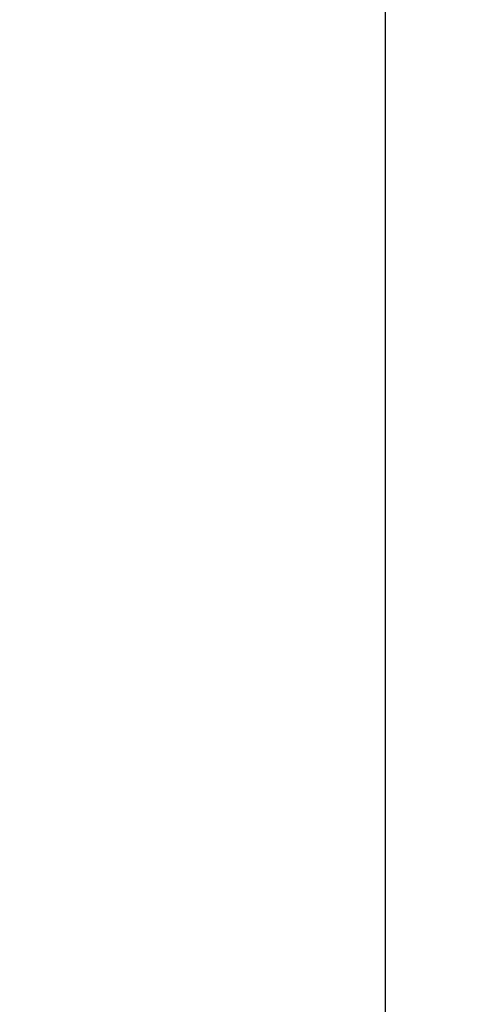
# Model space of a CAD drawing. Units: inches. Extents: x 1704 to 6393, y -157 to 1172.
# Tile 96 of 122: x 2750 to 2793, y 880 to 972. Entities that reach past the tile are written whole.
import ezdxf

# ---------------------------------------------------------------- set-up
doc = ezdxf.new("R2010")
doc.units = ezdxf.units.IN
doc.header["$MEASUREMENT"] = 0
doc.layers.add('A-ANNO-DIMS', color=7, linetype='Continuous', lineweight=13)
doc.styles.get("Standard").update_dxf_attribs({"font": 'arial.ttf'})
doc.dimstyles.get("Standard").update_dxf_attribs({"dimtxt": 6, "dimasz": 2, "dimexe": 0.18, "dimexo": 0.0625, "dimgap": 0.09, "dimtad": 0, "dimtih": 1, "dimtoh": 1, "dimdec": 1, "dimzin": 0, "dimdsep": 46, "dimlunit": 3, "dimtxsty": 'Standard', "dimblk": 'ARCHTICK', "dimcen": 0.09, "dimadec": 0, "dimazin": 0, "dimtfac": 1, "dimtdec": 1, "dimtofl": 0, "dimtmove": 0, "dimatfit": 3, "dimfxl": 1, "dimtolj": 1, "dimtzin": 0, "dimarcsym": 0})

# ---------------------------------------------------------------- blocks, each defined once
blk = doc.blocks.new('_ArchTick')
at = {"color": 0, "linetype": 'ByBlock', "const_width": 0.15}
blk.add_lwpolyline([(-0.5, -0.5), (0.5, 0.5)], dxfattribs=at)
blk = doc.blocks.new('*D91')
at = {"layer": 'A-ANNO-DIMS', "color": 0, "lineweight": -2, "transparency": 16777216}
for p, q in [((2723.411, 1033.213), (2784.529, 1033.213)), ((2784.349, 1033.213), (2784.349, 517.868)), ((2784.349, -3.787), (2784.349, 511.557)), ((2723.411, -3.787), (2784.529, -3.787))]:
    blk.add_line(p, q, dxfattribs=at)
at = {"layer": 'Defpoints', "color": 0, "lineweight": -3, "transparency": 16777216}
for p in [(2723.349, 1033.213), (2784.349, 1033.213), (2723.349, -3.787)]:
    blk.add_point(p, dxfattribs=at)
at = {"layer": 'A-ANNO-DIMS', "color": 0, "lineweight": -2, "transparency": 16777216, "xscale": 2, "yscale": 2, "zscale": 2}
for p, rotation in [((2784.349, 1033.213), 90), ((2784.349, -3.787), 270)]:
    blk.add_blockref('_ArchTick', p, dxfattribs=dict(at, rotation=rotation))
at = {"layer": 'A-ANNO-DIMS', "color": 0, "transparency": 16777216, "insert": (2784.349, 514.713), "char_height": 6, "attachment_point": 5}
blk.add_mtext('\\A1;1037', dxfattribs=at)

msp = doc.modelspace()

# ---------------------------------------------------------------- dimensions: what is measured, and where the dimension line sits
at = {"layer": 'A-ANNO-DIMS'}
dim = msp.add_linear_dim(base=(2784.349, 1033.213), p1=(2723.349, -3.787), p2=(2723.349, 1033.213), angle=90, dimstyle='Standard', override={"dimdec": 0, "dimlfac": 1, "dimrnd": 0, "dimzin": 0, "dimdsep": 46, "dimlunit": 2}, dxfattribs=at)
dim.commit()
dim.dimension.update_dxf_attribs({"geometry": '*D91', "text_midpoint": (2784.349, 514.713)})

doc.saveas('drawing.dxf')
